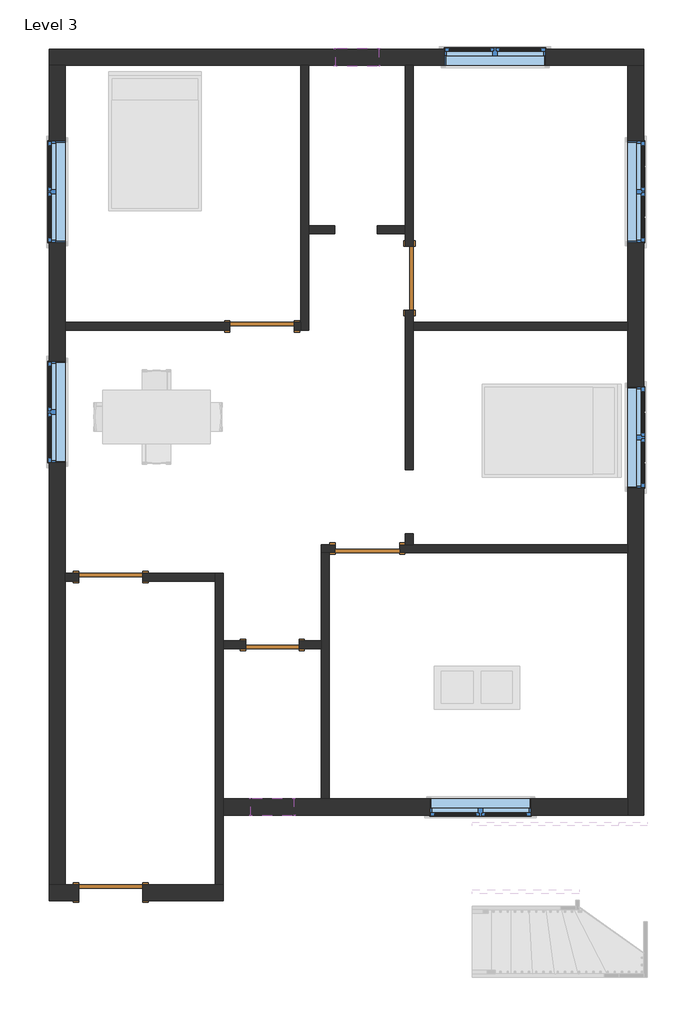
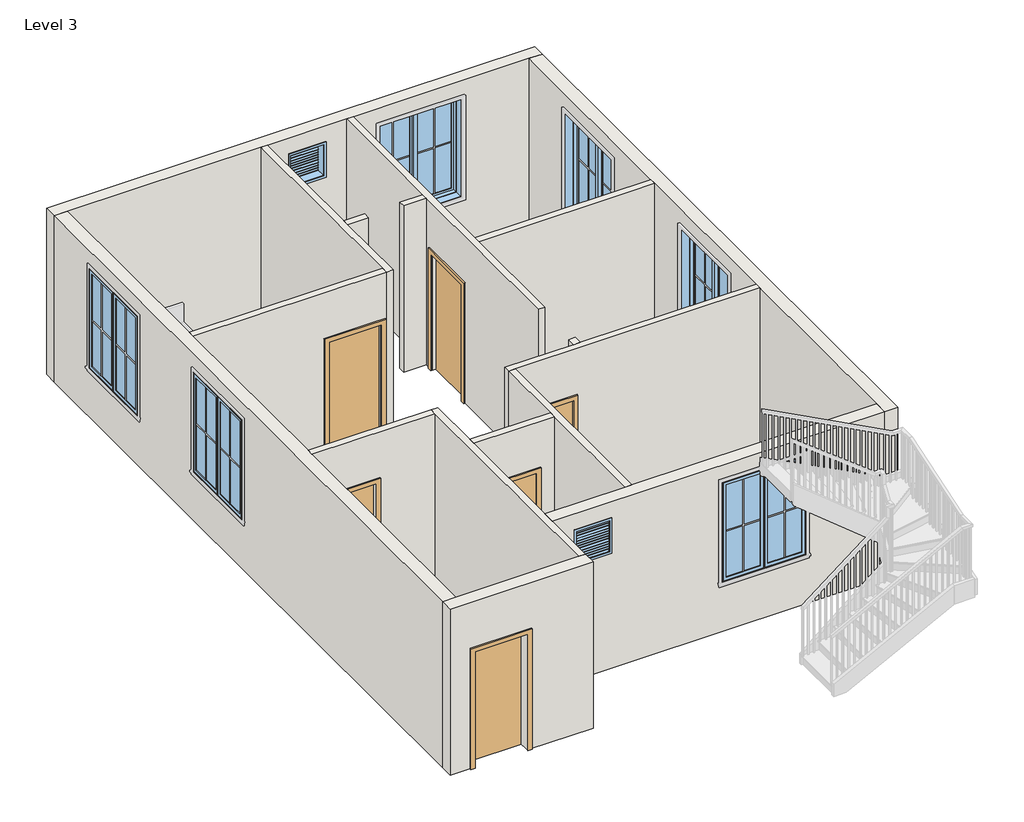
# One storey, part 1 of 3: 17 walls, 8 windows, 6 doors.
"""IFC4 building model written with IfcOpenShell, lengths in millimetres."""

from ifc_helpers import new_model, si_unit, frame, origin, place, context, project, spatial, polyline, outline, extrude, faceted_brep, transform, mapped, element, save
from components import door_214872d5, single_flush_door_3_e5f9f3c4, single_flush_door_3_305aa2a5, single_flush_door_3_a90ba1ad, window_9ac97e1a, window_f2d8fef0

model = new_model("IFC4")

# Units and contexts
model_context = context("Model", 3, world=origin())
ifc_project = project(units=[si_unit("LENGTHUNIT", "METRE", prefix="MILLI")], contexts=[model_context])

# Site, building, storey
site = spatial("IfcSite", under=ifc_project)
building = spatial("IfcBuilding", under=site)
storey = spatial("IfcBuildingStorey", under=building, Name="Level 3", Elevation=3200.4)

# Doors
placement = place(None, origin())
door_shape = door_214872d5(model_context)
element("IfcDoor", 1, ObjectType="Single-Flush : DOOR 2'6\"", at=placement, inside=storey, context=model_context, shape_type="MappedRepresentation", body=[
    mapped(door_shape, transform((-2309.3144966, -2885.2590409, 3200.4), x_axis=(-1.0, 0.0, 0.0), y_axis=(0.0, -1.0, 0.0), z_axis=(0.0, 0.0, 1.0))),
])
single_flush_door_3_shape = single_flush_door_3_e5f9f3c4(model_context)
element("IfcDoor", 2, ObjectType="Single-Flush : DOOR 3'", at=placement, inside=storey, context=model_context, shape_type="MappedRepresentation", body=[
    mapped(single_flush_door_3_shape, transform((-2455.3644966, 1648.6409591, 3200.4), x_axis=(1.0, 0.0, 0.0), y_axis=(0.0, 1.0, 0.0), z_axis=(0.0, 0.0, 1.0))),
])
element("IfcDoor", 3, ObjectType="Single-Flush : DOOR 3'", at=placement, inside=storey, context=model_context, shape_type="MappedRepresentation", body=[
    mapped(single_flush_door_3_shape, transform((-359.8644966, 2334.4409591, 3200.4), x_axis=(0.0, -1.0, 0.0), y_axis=(1.0, 0.0, 0.0), z_axis=(0.0, 0.0, 1.0))),
])
element("IfcDoor", 4, ObjectType="Single-Flush : DOOR 3'", at=placement, inside=storey, context=model_context, shape_type="MappedRepresentation", body=[
    mapped(single_flush_door_3_shape, transform((-956.7644966, -1513.6590409, 3200.4), x_axis=(-1.0, 0.0, 0.0), y_axis=(0.0, -1.0, 0.0), z_axis=(0.0, 0.0, 1.0))),
])
single_flush_door_3_2_shape = single_flush_door_3_305aa2a5(model_context)
element("IfcDoor", 5, ObjectType="Single-Flush : DOOR 3'", at=placement, inside=storey, context=model_context, shape_type="MappedRepresentation", body=[
    mapped(single_flush_door_3_2_shape, transform((-4608.0144966, -1920.0590409, 3200.4), x_axis=(-1.0, 0.0, 0.0), y_axis=(0.0, -1.0, 0.0), z_axis=(0.0, 0.0, 1.0))),
])
single_flush_door_3_3_shape = single_flush_door_3_a90ba1ad(model_context)
element("IfcDoor", 6, ObjectType="Single-Flush : DOOR 3'", at=placement, inside=storey, context=model_context, shape_type="MappedRepresentation", body=[
    mapped(single_flush_door_3_3_shape, transform((-4608.0144966, -6409.5090409, 3200.4), x_axis=(-1.0, 0.0, 0.0), y_axis=(0.0, -1.0, 0.0), z_axis=(0.0, 0.0, 1.0))),
])

# Walls
element("IfcWall", 7, ObjectType="WALL 4.5\"", at=placement, inside=storey, context=model_context, shape_type="Brep", body=[
    faceted_brep([(-1902.9144966, 5363.3909591, 3200.4), (-1902.9144966, 1705.7909591, 3200.4), (-1902.9144966, 1591.4909591, 3200.4), (-1902.9144966, 1591.4909591, 6248.4), (-1902.9144966, 1705.7909591, 6248.4), (-1902.9144966, 5363.3909591, 6248.4), (-1788.6144966, 5363.3909591, 3200.4), (-1788.6144966, 5363.3909591, 6248.4), (-1788.6144966, 3077.3909591, 6248.4), (-1788.6144966, 2963.0909591, 6248.4), (-1788.6144966, 1591.4909591, 6248.4), (-1788.6144966, 1591.4909591, 3200.4), (-1788.6144966, 2963.0909591, 3200.4), (-1788.6144966, 3077.3909591, 3200.4)], [[[0, 1, 2, 3, 4, 5]], [[6, 7, 8, 9, 10, 11, 12, 13]], [[2, 1, 0, 6, 13, 12, 11]], [[0, 5, 7, 6]], [[3, 2, 11, 10]], [[5, 4, 3, 10, 9, 8, 7]]]),
])
element("IfcWall", 8, ObjectType="WALL 4.5\"", at=placement, inside=storey, context=model_context, shape_type="SweptSolid", body=[
    extrude(outline(polyline([(5334.0, -1998.1644966), (3200.4, -1998.1644966), (3200.4, -1902.9144966), (6248.4, -1902.9144966), (6248.4, -5255.7144966), (3200.4, -5255.7144966), (3200.4, -2912.5644966), (5334.0, -2912.5644966), (5334.0, -1998.1644966)])), frame((0.0, 1591.4909591, 0.0), z_axis=(0.0, 1.0, 0.0), x_axis=(0.0, 0.0, 1.0)), (0.0, 0.0, 1.0), 114.3),
])
element("IfcWall", 9, ObjectType="WALL 4.5\"", at=placement, inside=storey, context=model_context, shape_type="Brep", body=[
    faceted_brep([(-417.0144966, 1877.2409591, 5334.0), (-417.0144966, 1877.2409591, 3200.4), (-417.0144966, -389.7090409, 3200.4), (-417.0144966, -389.7090409, 6248.4), (-417.0144966, 2963.0909591, 6248.4), (-417.0144966, 3077.3909591, 6248.4), (-417.0144966, 5363.3909591, 6248.4), (-417.0144966, 5363.3909591, 3200.4), (-417.0144966, 3077.3909591, 3200.4), (-417.0144966, 2963.0909591, 3200.4), (-417.0144966, 2791.6409591, 3200.4), (-417.0144966, 2791.6409591, 5334.0), (-302.7144966, -389.7090409, 3200.4), (-302.7144966, 1591.4909591, 3200.4), (-302.7144966, 1705.7909591, 3200.4), (-302.7144966, 1877.2409591, 3200.4), (-302.7144966, 1877.2409591, 5334.0), (-302.7144966, 2791.6409591, 5334.0), (-302.7144966, 2791.6409591, 3200.4), (-302.7144966, 5363.3909591, 3200.4), (-302.7144966, 5363.3909591, 6248.4), (-302.7144966, 1705.7909591, 6248.4), (-302.7144966, 1591.4909591, 6248.4), (-302.7144966, -389.7090409, 6248.4)], [[[0, 1, 2, 3, 4, 5, 6, 7, 8, 9, 10, 11]], [[12, 13, 14, 15, 16, 17, 18, 19, 20, 21, 22, 23]], [[2, 1, 15, 14, 13, 12]], [[10, 9, 8, 7, 19, 18]], [[3, 2, 12, 23]], [[7, 6, 20, 19]], [[16, 15, 1, 0]], [[17, 16, 0, 11]], [[18, 17, 11, 10]], [[6, 5, 4, 3, 23, 22, 21, 20]]]),
])
element("IfcWall", 10, ObjectType="WALL 4.5\"", at=placement, inside=storey, context=model_context, shape_type="SweptSolid", body=[
    extrude(outline(polyline([(-302.7144966, 1705.7909591), (2745.2855034, 1705.7909591), (2745.2855034, 1591.4909591), (-302.7144966, 1591.4909591), (-302.7144966, 1705.7909591)])), frame((0.0, 0.0, 3200.4), z_axis=(0.0, 0.0, 1.0), x_axis=(1.0, 0.0, 0.0)), (0.0, 0.0, 1.0), 3048.0),
])
element("IfcWall", 11, ObjectType="WALL 4.5\"", at=placement, inside=storey, context=model_context, shape_type="SweptSolid", body=[
    extrude(outline(polyline([(-1423.1234474, 2963.0909591), (-1788.6144966, 2963.0909591), (-1788.6144966, 3077.3909591), (-1423.1234474, 3077.3909591), (-1423.1234474, 2963.0909591)])), frame((0.0, 0.0, 3200.4), z_axis=(0.0, 0.0, 1.0), x_axis=(1.0, 0.0, 0.0)), (0.0, 0.0, 1.0), 3048.0),
])
element("IfcWall", 12, ObjectType="WALL 4.5\"", at=placement, inside=storey, context=model_context, shape_type="Brep", body=[
    faceted_brep([(-1413.9644966, -1456.5090409, 5334.0), (-1413.9644966, -1456.5090409, 3200.4), (-1610.8144966, -1456.5090409, 3200.4), (-1610.8144966, -1456.5090409, 6248.4), (-417.0144966, -1456.5090409, 6248.4), (-302.7144966, -1456.5090409, 6248.4), (2745.2855034, -1456.5090409, 6248.4), (2745.2855034, -1456.5090409, 3200.4), (-302.7144966, -1456.5090409, 3200.4), (-417.0144966, -1456.5090409, 3200.4), (-499.5644966, -1456.5090409, 3200.4), (-499.5644966, -1456.5090409, 5334.0), (-1610.8144966, -1570.8090409, 3200.4), (-1496.5144966, -1570.8090409, 3200.4), (-1413.9644966, -1570.8090409, 3200.4), (-1413.9644966, -1570.8090409, 5334.0), (-499.5644966, -1570.8090409, 5334.0), (-499.5644966, -1570.8090409, 3200.4), (2745.2855034, -1570.8090409, 3200.4), (2745.2855034, -1570.8090409, 6248.4), (-1496.5144966, -1570.8090409, 6248.4), (-1610.8144966, -1570.8090409, 6248.4)], [[[0, 1, 2, 3, 4, 5, 6, 7, 8, 9, 10, 11]], [[12, 13, 14, 15, 16, 17, 18, 19, 20, 21]], [[2, 1, 14, 13, 12]], [[10, 9, 8, 7, 18, 17]], [[7, 6, 19, 18]], [[3, 2, 12, 21]], [[15, 14, 1, 0]], [[16, 15, 0, 11]], [[17, 16, 11, 10]], [[6, 5, 4, 3, 21, 20, 19]]]),
])
element("IfcWall", 13, ObjectType="WALL 4.5\"", at=placement, inside=storey, context=model_context, shape_type="SweptSolid", body=[
    extrude(outline(polyline([(-302.7144966, -1304.1090409), (-302.7144966, -1456.5090409), (-417.0144966, -1456.5090409), (-417.0144966, -1304.1090409), (-302.7144966, -1304.1090409)])), frame((0.0, 0.0, 3200.4), z_axis=(0.0, 0.0, 1.0), x_axis=(1.0, 0.0, 0.0)), (0.0, 0.0, 1.0), 3048.0),
])
element("IfcWall", 14, ObjectType="WALL 4.5\"", at=placement, inside=storey, context=model_context, shape_type="Brep", body=[
    faceted_brep([(-1610.8144966, -1570.8090409, 3200.4), (-1610.8144966, -2828.1090409, 3200.4), (-1610.8144966, -2942.4090409, 3200.4), (-1610.8144966, -5076.0090409, 3200.4), (-1610.8144966, -5076.0090409, 6248.4), (-1610.8144966, -2942.4090409, 6248.4), (-1610.8144966, -2828.1090409, 6248.4), (-1610.8144966, -1570.8090409, 6248.4), (-1496.5144966, -1570.8090409, 3200.4), (-1496.5144966, -1570.8090409, 6248.4), (-1496.5144966, -5076.0090409, 6248.4), (-1496.5144966, -5076.0090409, 3200.4)], [[[0, 1, 2, 3, 4, 5, 6, 7]], [[8, 9, 10, 11]], [[3, 2, 1, 0, 8, 11]], [[0, 7, 9, 8]], [[4, 3, 11, 10]], [[7, 6, 5, 4, 10, 9]]]),
])
element("IfcWall", 15, ObjectType="WALL 4.5\"", at=placement, inside=storey, context=model_context, shape_type="SweptSolid", body=[
    extrude(outline(polyline([(3200.4, -3007.8144966), (3200.4, -2690.3144966), (5334.0, -2690.3144966), (5334.0, -1928.3144966), (3200.4, -1928.3144966), (3200.4, -1610.8144966), (6248.4, -1610.8144966), (6248.4, -3007.8144966), (3200.4, -3007.8144966)])), frame((0.0, -2942.4090409, 0.0), z_axis=(0.0, 1.0, 0.0), x_axis=(0.0, 0.0, 1.0)), (0.0, 0.0, 1.0), 114.3),
])
element("IfcWall", 16, ObjectType="WALL 4.5\"", at=placement, inside=storey, context=model_context, shape_type="Brep", body=[
    faceted_brep([(-3007.8144966, -6295.2090409, 3200.4), (-3007.8144966, -5304.6090409, 3200.4), (-3007.8144966, -5076.0090409, 3200.4), (-3007.8144966, -2942.4090409, 3200.4), (-3007.8144966, -2828.1090409, 3200.4), (-3007.8144966, -1862.9090409, 3200.4), (-3007.8144966, -1862.9090409, 6248.4), (-3007.8144966, -2828.1090409, 6248.4), (-3007.8144966, -2942.4090409, 6248.4), (-3007.8144966, -5076.0090409, 6248.4), (-3007.8144966, -5304.6090409, 6248.4), (-3007.8144966, -6295.2090409, 6248.4), (-3122.1144966, -6295.2090409, 3200.4), (-3122.1144966, -6295.2090409, 6248.4), (-3122.1144966, -1977.2090409, 6248.4), (-3122.1144966, -1862.9090409, 6248.4), (-3122.1144966, -1862.9090409, 3200.4), (-3122.1144966, -1977.2090409, 3200.4)], [[[0, 1, 2, 3, 4, 5, 6, 7, 8, 9, 10, 11]], [[12, 13, 14, 15, 16, 17]], [[5, 4, 3, 2, 1, 0, 12, 17, 16]], [[0, 11, 13, 12]], [[6, 5, 16, 15]], [[11, 10, 9, 8, 7, 6, 15, 14, 13]]]),
])
element("IfcWall", 17, ObjectType="WALL 4.5\"", at=placement, inside=storey, context=model_context, shape_type="SweptSolid", body=[
    extrude(outline(polyline([(3200.4, -5255.7144966), (3200.4, -5065.2144966), (5334.0, -5065.2144966), (5334.0, -4150.8144966), (3200.4, -4150.8144966), (3200.4, -3122.1144966), (6248.4, -3122.1144966), (6248.4, -5255.7144966), (3200.4, -5255.7144966)])), frame((0.0, -1977.2090409, 0.0), z_axis=(0.0, 1.0, 0.0), x_axis=(0.0, 0.0, 1.0)), (0.0, 0.0, 1.0), 114.3),
])
element("IfcWall", 18, ObjectType="WALL 4.5\"", at=placement, inside=storey, context=model_context, shape_type="SweptSolid", body=[
    extrude(outline(polyline([(-417.0144966, 2963.0909591), (-814.3659123, 2963.0909591), (-814.3659123, 3077.3909591), (-417.0144966, 3077.3909591), (-417.0144966, 2963.0909591)])), frame((0.0, 0.0, 3200.4), z_axis=(0.0, 0.0, 1.0), x_axis=(1.0, 0.0, 0.0)), (0.0, 0.0, 1.0), 3048.0),
])
element("IfcWall", 19, ObjectType="WALL 9\"", at=placement, inside=storey, context=model_context, shape_type="Brep", body=[
    faceted_brep([(-5484.3144966, 5363.3909591, 3200.4), (-5255.7144966, 5363.3909591, 3200.4), (-1902.9144966, 5363.3909591, 3200.4), (-1788.6144966, 5363.3909591, 3200.4), (-417.0144966, 5363.3909591, 3200.4), (-302.7144966, 5363.3909591, 3200.4), (2745.2855034, 5363.3909591, 3200.4), (2973.8855034, 5363.3909591, 3200.4), (2973.8855034, 5363.3909591, 6248.4), (2745.2855034, 5363.3909591, 6248.4), (-302.7144966, 5363.3909591, 6248.4), (-417.0144966, 5363.3909591, 6248.4), (-1788.6144966, 5363.3909591, 6248.4), (-1902.9144966, 5363.3909591, 6248.4), (-5255.7144966, 5363.3909591, 6248.4), (-5484.3144966, 5363.3909591, 6248.4), (1583.2355034, 5363.3909591, 5943.6), (1583.2355034, 5363.3909591, 4114.8), (135.4355034, 5363.3909591, 4114.8), (135.4355034, 5363.3909591, 5943.6), (-1407.6144966, 5363.3909591, 5943.6), (-798.0144966, 5363.3909591, 5943.6), (-798.0144966, 5363.3909591, 5334.0), (-1407.6144966, 5363.3909591, 5334.0), (-5484.3144966, 5591.9909591, 3200.4), (-5484.3144966, 5591.9909591, 6248.4), (2973.8855034, 5591.9909591, 6248.4), (2973.8855034, 5591.9909591, 3200.4), (1583.2355034, 5591.9909591, 5943.6), (135.4355034, 5591.9909591, 5943.6), (135.4355034, 5591.9909591, 4114.8), (1583.2355034, 5591.9909591, 4114.8), (-1407.6144966, 5591.9909591, 5943.6), (-1407.6144966, 5591.9909591, 5334.0), (-798.0144966, 5591.9909591, 5334.0), (-798.0144966, 5591.9909591, 5943.6)], [[[0, 1, 2, 3, 4, 5, 6, 7, 8, 9, 10, 11, 12, 13, 14, 15], [16, 17, 18, 19], [20, 21, 22, 23]], [[24, 25, 26, 27], [28, 29, 30, 31], [32, 33, 34, 35]], [[7, 6, 5, 4, 3, 2, 1, 0, 24, 27]], [[8, 7, 27, 26]], [[0, 15, 25, 24]], [[17, 16, 28, 31]], [[18, 17, 31, 30]], [[19, 18, 30, 29]], [[16, 19, 29, 28]], [[33, 32, 20, 23]], [[34, 33, 23, 22]], [[35, 34, 22, 21]], [[32, 35, 21, 20]], [[15, 14, 13, 12, 11, 10, 9, 8, 26, 25]]]),
])
element("IfcWall", 20, ObjectType="WALL 9\"", at=placement, inside=storey, context=model_context, shape_type="Brep", body=[
    faceted_brep([(2745.2855034, 5363.3909591, 3200.4), (2745.2855034, 1705.7909591, 3200.4), (2745.2855034, 1591.4909591, 3200.4), (2745.2855034, -1456.5090409, 3200.4), (2745.2855034, -1570.8090409, 3200.4), (2745.2855034, -5076.0090409, 3200.4), (2745.2855034, -5304.6090409, 3200.4), (2745.2855034, -5304.6090409, 6248.4), (2745.2855034, -5076.0090409, 6248.4), (2745.2855034, -1570.8090409, 6248.4), (2745.2855034, -1456.5090409, 6248.4), (2745.2855034, 1591.4909591, 6248.4), (2745.2855034, 1705.7909591, 6248.4), (2745.2855034, 5363.3909591, 6248.4), (2745.2855034, -656.4090409, 5943.6), (2745.2855034, -656.4090409, 4114.8), (2745.2855034, 791.3909591, 4114.8), (2745.2855034, 791.3909591, 5943.6), (2745.2855034, 2839.2659591, 5943.6), (2745.2855034, 2839.2659591, 4114.8), (2745.2855034, 4287.0659591, 4114.8), (2745.2855034, 4287.0659591, 5943.6), (2973.8855034, 5363.3909591, 3200.4), (2973.8855034, 5363.3909591, 6248.4), (2973.8855034, -5304.6090409, 6248.4), (2973.8855034, -5304.6090409, 3200.4), (2973.8855034, -656.4090409, 5943.6), (2973.8855034, 791.3909591, 5943.6), (2973.8855034, 791.3909591, 4114.8), (2973.8855034, -656.4090409, 4114.8), (2973.8855034, 2839.2659591, 5943.6), (2973.8855034, 4287.0659591, 5943.6), (2973.8855034, 4287.0659591, 4114.8), (2973.8855034, 2839.2659591, 4114.8)], [[[0, 1, 2, 3, 4, 5, 6, 7, 8, 9, 10, 11, 12, 13], [14, 15, 16, 17], [18, 19, 20, 21]], [[22, 23, 24, 25], [26, 27, 28, 29], [30, 31, 32, 33]], [[6, 5, 4, 3, 2, 1, 0, 22, 25]], [[0, 13, 23, 22]], [[7, 6, 25, 24]], [[15, 14, 26, 29]], [[16, 15, 29, 28]], [[17, 16, 28, 27]], [[14, 17, 27, 26]], [[19, 18, 30, 33]], [[20, 19, 33, 32]], [[21, 20, 32, 31]], [[18, 21, 31, 30]], [[13, 12, 11, 10, 9, 8, 7, 24, 23]]]),
])
element("IfcWall", 21, ObjectType="WALL 9\"", at=placement, inside=storey, context=model_context, shape_type="Brep", body=[
    faceted_brep([(2745.2855034, -5076.0090409, 3200.4), (-1496.5144966, -5076.0090409, 3200.4), (-1610.8144966, -5076.0090409, 3200.4), (-3007.8144966, -5076.0090409, 3200.4), (-3007.8144966, -5076.0090409, 6248.4), (-1610.8144966, -5076.0090409, 6248.4), (-1496.5144966, -5076.0090409, 6248.4), (2745.2855034, -5076.0090409, 6248.4), (-70.9394966, -5076.0090409, 5943.6), (-70.9394966, -5076.0090409, 4114.8), (1376.8605034, -5076.0090409, 4114.8), (1376.8605034, -5076.0090409, 5943.6), (-2004.5144966, -5076.0090409, 5943.6), (-2614.1144966, -5076.0090409, 5943.6), (-2614.1144966, -5076.0090409, 5334.0), (-2004.5144966, -5076.0090409, 5334.0), (2745.2855034, -5304.6090409, 3200.4), (2745.2855034, -5304.6090409, 6248.4), (-3007.8144966, -5304.6090409, 6248.4), (-3007.8144966, -5304.6090409, 3200.4), (-70.9394966, -5304.6090409, 5943.6), (1376.8605034, -5304.6090409, 5943.6), (1376.8605034, -5304.6090409, 4114.8), (-70.9394966, -5304.6090409, 4114.8), (-2004.5144966, -5304.6090409, 5943.6), (-2004.5144966, -5304.6090409, 5334.0), (-2614.1144966, -5304.6090409, 5334.0), (-2614.1144966, -5304.6090409, 5943.6)], [[[0, 1, 2, 3, 4, 5, 6, 7], [8, 9, 10, 11], [12, 13, 14, 15]], [[16, 17, 18, 19], [20, 21, 22, 23], [24, 25, 26, 27]], [[3, 2, 1, 0, 16, 19]], [[0, 7, 17, 16]], [[4, 3, 19, 18]], [[9, 8, 20, 23]], [[10, 9, 23, 22]], [[11, 10, 22, 21]], [[8, 11, 21, 20]], [[25, 24, 12, 15]], [[26, 25, 15, 14]], [[27, 26, 14, 13]], [[24, 27, 13, 12]], [[7, 6, 5, 4, 18, 17]]]),
])
element("IfcWall", 22, ObjectType="WALL 9\"", at=placement, inside=storey, context=model_context, shape_type="Brep", body=[
    faceted_brep([(-5065.2144966, -6295.2090409, 5334.0), (-5065.2144966, -6295.2090409, 3200.4), (-5255.7144966, -6295.2090409, 3200.4), (-5484.3144966, -6295.2090409, 3200.4), (-5484.3144966, -6295.2090409, 6248.4), (-5255.7144966, -6295.2090409, 6248.4), (-3122.1144966, -6295.2090409, 6248.4), (-3007.8144966, -6295.2090409, 6248.4), (-3007.8144966, -6295.2090409, 3200.4), (-3122.1144966, -6295.2090409, 3200.4), (-4150.8144966, -6295.2090409, 3200.4), (-4150.8144966, -6295.2090409, 5334.0), (-5484.3144966, -6523.8090409, 3200.4), (-5065.2144966, -6523.8090409, 3200.4), (-5065.2144966, -6523.8090409, 5334.0), (-4150.8144966, -6523.8090409, 5334.0), (-4150.8144966, -6523.8090409, 3200.4), (-3007.8144966, -6523.8090409, 3200.4), (-3007.8144966, -6523.8090409, 6248.4), (-5484.3144966, -6523.8090409, 6248.4)], [[[0, 1, 2, 3, 4, 5, 6, 7, 8, 9, 10, 11]], [[12, 13, 14, 15, 16, 17, 18, 19]], [[10, 9, 8, 17, 16]], [[3, 2, 1, 13, 12]], [[4, 3, 12, 19]], [[8, 7, 18, 17]], [[7, 6, 5, 4, 19, 18]], [[14, 13, 1, 0]], [[15, 14, 0, 11]], [[16, 15, 11, 10]]]),
])
element("IfcWall", 23, ObjectType="WALL 9\"", at=placement, inside=storey, context=model_context, shape_type="Brep", body=[
    faceted_brep([(-5255.7144966, -6295.2090409, 3200.4), (-5255.7144966, -1977.2090409, 3200.4), (-5255.7144966, -1862.9090409, 3200.4), (-5255.7144966, 1591.4909591, 3200.4), (-5255.7144966, 1705.7909591, 3200.4), (-5255.7144966, 5363.3909591, 3200.4), (-5255.7144966, 5363.3909591, 6248.4), (-5255.7144966, 1705.7909591, 6248.4), (-5255.7144966, 1591.4909591, 6248.4), (-5255.7144966, -1862.9090409, 6248.4), (-5255.7144966, -1977.2090409, 6248.4), (-5255.7144966, -6295.2090409, 6248.4), (-5255.7144966, 4287.0659591, 5943.6), (-5255.7144966, 4287.0659591, 4114.8), (-5255.7144966, 2839.2659591, 4114.8), (-5255.7144966, 2839.2659591, 5943.6), (-5255.7144966, 1153.3409591, 5943.6), (-5255.7144966, 1153.3409591, 4114.8), (-5255.7144966, -294.4590409, 4114.8), (-5255.7144966, -294.4590409, 5943.6), (-5484.3144966, -6295.2090409, 3200.4), (-5484.3144966, -6295.2090409, 6248.4), (-5484.3144966, 5363.3909591, 6248.4), (-5484.3144966, 5363.3909591, 3200.4), (-5484.3144966, 4287.0659591, 5943.6), (-5484.3144966, 2839.2659591, 5943.6), (-5484.3144966, 2839.2659591, 4114.8), (-5484.3144966, 4287.0659591, 4114.8), (-5484.3144966, 1153.3409591, 5943.6), (-5484.3144966, -294.4590409, 5943.6), (-5484.3144966, -294.4590409, 4114.8), (-5484.3144966, 1153.3409591, 4114.8)], [[[0, 1, 2, 3, 4, 5, 6, 7, 8, 9, 10, 11], [12, 13, 14, 15], [16, 17, 18, 19]], [[20, 21, 22, 23], [24, 25, 26, 27], [28, 29, 30, 31]], [[5, 4, 3, 2, 1, 0, 20, 23]], [[0, 11, 21, 20]], [[6, 5, 23, 22]], [[13, 12, 24, 27]], [[14, 13, 27, 26]], [[15, 14, 26, 25]], [[12, 15, 25, 24]], [[17, 16, 28, 31]], [[18, 17, 31, 30]], [[19, 18, 30, 29]], [[16, 19, 29, 28]], [[11, 10, 9, 8, 7, 6, 22, 21]]]),
])

# Windows
window_shape = window_9ac97e1a(model_context)
element("IfcWindow", 24, ObjectType="Window-Casement-Double : 57\" x 72\"", at=placement, inside=storey, context=model_context, shape_type="MappedRepresentation", body=[
    mapped(window_shape, transform((2859.5855034, 67.4909591, 3200.4), x_axis=(0.0, -1.0, 0.0), y_axis=(1.0, 0.0, 0.0), z_axis=(0.0, 0.0, 1.0))),
])
element("IfcWindow", 25, ObjectType="Window-Casement-Double : 57\" x 72\"", at=placement, inside=storey, context=model_context, shape_type="MappedRepresentation", body=[
    mapped(window_shape, transform((2859.5855034, 3563.1659591, 3200.4), x_axis=(0.0, -1.0, 0.0), y_axis=(1.0, 0.0, 0.0), z_axis=(0.0, 0.0, 1.0))),
])
element("IfcWindow", 26, ObjectType="Window-Casement-Double : 57\" x 72\"", at=placement, inside=storey, context=model_context, shape_type="MappedRepresentation", body=[
    mapped(window_shape, transform((859.3355034, 5477.6909591, 3200.4), x_axis=(1.0, 0.0, 0.0), y_axis=(0.0, 1.0, 0.0), z_axis=(0.0, 0.0, 1.0))),
])
element("IfcWindow", 27, ObjectType="Window-Casement-Double : 57\" x 72\"", at=placement, inside=storey, context=model_context, shape_type="MappedRepresentation", body=[
    mapped(window_shape, transform((-5370.0144966, 3563.1659591, 3200.4), x_axis=(0.0, 1.0, 0.0), y_axis=(-1.0, 0.0, 0.0), z_axis=(0.0, 0.0, 1.0))),
])
element("IfcWindow", 28, ObjectType="Window-Casement-Double : 57\" x 72\"", at=placement, inside=storey, context=model_context, shape_type="MappedRepresentation", body=[
    mapped(window_shape, transform((-5370.0144966, 429.4409591, 3200.4), x_axis=(0.0, 1.0, 0.0), y_axis=(-1.0, 0.0, 0.0), z_axis=(0.0, 0.0, 1.0))),
])
element("IfcWindow", 29, ObjectType="Window-Casement-Double : 57\" x 72\"", at=placement, inside=storey, context=model_context, shape_type="MappedRepresentation", body=[
    mapped(window_shape, transform((652.9605034, -5190.3090409, 3200.4), x_axis=(-1.0, 0.0, 0.0), y_axis=(0.0, -1.0, 0.0), z_axis=(0.0, 0.0, 1.0))),
])
window_2_shape = window_f2d8fef0(model_context)
element("IfcWindow", 30, ObjectType="Window-Louvers : 24\" x 24\"", at=placement, inside=storey, context=model_context, shape_type="MappedRepresentation", body=[
    mapped(window_2_shape, transform((-1102.8144966, 5484.0409591, 4419.6), x_axis=(1.0, 0.0, 0.0), y_axis=(0.0, 1.0, 0.0), z_axis=(0.0, 0.0, 1.0))),
])
element("IfcWindow", 31, ObjectType="Window-Louvers : 24\" x 24\"", at=placement, inside=storey, context=model_context, shape_type="MappedRepresentation", body=[
    mapped(window_2_shape, transform((-2309.3144966, -5196.6590409, 4419.6), x_axis=(-1.0, 0.0, 0.0), y_axis=(0.0, -1.0, 0.0), z_axis=(0.0, 0.0, 1.0))),
])

save(model, "model.ifc")

# Revit data of these elements
# Type "Single-Flush : DOOR 2'6\""
#   Type Mark = "10"
#   Construction Type Id = "MDOOR"
#   Assembly Code = "C1020"
#   Analytic Construction = "Metal"
#   Thickness = 0' - 2"
#   Heat Transfer Coefficient (U) = 0.651978 BTU/(h·ft²·°F)
#   Height = 7' - 0"
#   Trim Projection Ext = 0' - 1"
#   Trim Projection Int = 0' - 1"
#   Trim Width = 0' - 3"
#   Width = 2' - 6"
#   Define Thermal Properties by = 1
#   Door Material = Door - Panel
#   Frame Material = Door - Frame
#   Visual Light Transmittance = 0
#   Solar Heat Gain Coefficient = 0
#   Function = (empty or 0)
#   Wall Closure = (empty or 0)
# Type "Single-Flush : DOOR 3'"
#   Type Mark = "9"
#   Construction Type Id = "MDOOR"
#   Assembly Code = "C1020"
#   Analytic Construction = "Metal"
#   Thickness = 0' - 2"
#   Heat Transfer Coefficient (U) = 0.651978 BTU/(h·ft²·°F)
#   Height = 7' - 0"
#   Trim Projection Ext = 0' - 1"
#   Trim Projection Int = 0' - 1"
#   Trim Width = 0' - 3"
#   Width = 3' - 0"
#   Define Thermal Properties by = 1
#   Door Material = Door - Panel
#   Frame Material = Door - Frame
#   Visual Light Transmittance = 0
#   Solar Heat Gain Coefficient = 0
#   Function = (empty or 0)
#   Wall Closure = (empty or 0)
# Type "WALL 4.5\""
#   Assembly Code = "B2010"
#   Layers, outside or top first: 0' - 4 1/2" no material (function 1)
# Type "WALL 9\""
#   Assembly Code = "B2010"
#   Layers, outside or top first: 0' - 9" no material (function 1)
# Type "Window-Casement-Double : 57\" x 72\""
#   Type Mark = "17"
#   Fire Rating = "0.5h"
#   Assembly Code = "B2020100"
#   Analytic Construction = "Double glazing - domestic"
#   Frame Extension [instance default] = 0' - 0 1/4"
#   Window Inset [instance default] = 0' - 0"
#   Wall Thickness [instance default] = 0' - 6"
#   Interior Wall Closure [instance default] = 0' - 2 1/4"
#   Half Width = 2' - 4 1/2"
#   Visual Light Transmittance = 0.81
#   Thermal Resistance (R) = 1.8146 (h·ft²·°F)/BTU
#   Solar Heat Gain Coefficient = 0.76
#   Rough Width = 4' - 9 1/2"
#   Rough Height = 6' - 0 1/2"
#   Height = 6' - 0"
#   Heat Transfer Coefficient (U) = 0.5511 BTU/(h·ft²·°F)
#   Exterior Wall Closure [instance default] = 0' - 1 1/4"
#   Extension Jamb [instance default] = 0' - 2 1/4"
#   Default Sill Height = 3' - 0"
#   Width = 4' - 9"
#   Define Thermal Properties by = 0
#   Muntin Visibility = yes
#   Interior Trim Visibility [instance default] = yes
#   Exterior Trim Visibility [instance default] = yes
#   Extension Jamb Visibility [instance default] = yes
#   Interior Trim Material = Wood - Stained
#   Muntin Pattern = Muntin Pattern_2x2 : Muntin Pattern_2x2
#   Interior Trim = Trim-Window-Interior-Flat : Picture Frame
#   Interior Frame Material = Wood - Stained
#   Glass Panel Material = Glass
#   Exterior Trim Material = Clad - White
#   Exterior Trim = Trim-Window-Exterior-Flat : with Sill
#   Exterior Frame Material = Clad - White
#   Wall Closure = (empty or 0)
# Type "Window-Louvers : 24\" x 24\""
#   Type Mark = "18"
#   Construction Type Id = "GSP4R"
#   Assembly Code = "B20"
#   Analytic Construction = "1/8 in Pilkington single glazing"
#   Visual Light Transmittance = 0.9
#   Thermal Resistance (R) = 1.53941 (h·ft²·°F)/BTU
#   Solar Heat Gain Coefficient = 0.78
#   Max Height = 1' - 11.74264"
#   Height = 2' - 0"
#   Heat Transfer Coefficient (U) = 0.6496 BTU/(h·ft²·°F)
#   Blade Width [instance default] = 1' - 10 1/2"
#   Blade Vertical Thickness = 0' - 0.35355"
#   Blade Thickness = 0' - 0 1/4"
#   Blade Spacing = 0' - 1 1/2"
#   Blade Height = 0' - 1.85355"
#   Blade Depth = 0' - 3"
#   Blade Angle = 45.00°
#   Default Sill Height = 3' - 0"
#   Trim Projection_Exterior = 0' - 0 1/2"
#   Trim Projection_Interior = 0' - 0 1/2"
#   Trim Width_Exterior = 0' - 1 1/2"
#   Trim Width_Interior = 0' - 1 1/2"
#   Width = 2' - 0"
#   Max Blade Count = 12
#   Define Thermal Properties by = 1
#   Blade Count = 12
#   Frame Material = Birch
#   Louver Material = Birch
#   Trim Exterior Material = Birch
#   Trim Interior Material = Birch
#   Wall Closure = (empty or 0)
# Element 1 (IfcDoor, "Single-Flush : DOOR 2'6\"")
#   Phase Created = New Construction
#   Materials on its faces: "Door - Frame", "Door - Panel"
# Elements 2, 3, 4, 5, 6 (IfcDoor, "Single-Flush : DOOR 3'")
#   Phase Created = New Construction
#   Materials on its faces: "Door - Frame", "Door - Panel"
# Elements 7, 8, 9, 10, 11, 12, 13, 14, 15, 16, 17, 18 (IfcWall, "WALL 4.5\"")
#   Top Offset = 0' - 0"
#   Base Offset = 0' - 0"
#   Unconnected Height = 10' - 0"
#   wall height = 10' - 0"
#   Phase Created = New Construction
#   Base Constraint = Level 3
#   Materials on its faces: "Default Wall"
# Elements 19, 20, 21, 22, 23 (IfcWall, "WALL 9\"")
#   Top Offset = 0' - 0"
#   Base Offset = 0' - 0"
#   Unconnected Height = 10' - 0"
#   wall height = 10' - 0"
#   Phase Created = New Construction
#   Base Constraint = Level 3
#   Materials on its faces: "Default Wall"
# Element 24 (IfcWindow, "Window-Casement-Double : 57\" x 72\"")
#   Mark = "9"
#   Window Inset = 0' - 0"
#   Interior Wall Closure = 0' - 2 1/4"
#   Frame Extension = 0' - 0 1/4"
#   Exterior Wall Closure = 0' - 1 1/4"
#   Interior Trim Visibility = yes
#   Exterior Trim Visibility = yes
#   Phase Created = New Construction
#   Materials on its faces: "Wood - Stained", "Glass", "Clad - White"
# Element 25 (IfcWindow, "Window-Casement-Double : 57\" x 72\"")
#   Mark = "10"
#   Window Inset = 0' - 0"
#   Interior Wall Closure = 0' - 2 1/4"
#   Frame Extension = 0' - 0 1/4"
#   Exterior Wall Closure = 0' - 1 1/4"
#   Interior Trim Visibility = yes
#   Exterior Trim Visibility = yes
#   Phase Created = New Construction
#   Materials on its faces: "Wood - Stained", "Glass", "Clad - White"
# Element 26 (IfcWindow, "Window-Casement-Double : 57\" x 72\"")
#   Mark = "11"
#   Window Inset = 0' - 0"
#   Interior Wall Closure = 0' - 2 1/4"
#   Frame Extension = 0' - 0 1/4"
#   Exterior Wall Closure = 0' - 1 1/4"
#   Interior Trim Visibility = yes
#   Exterior Trim Visibility = yes
#   Phase Created = New Construction
#   Materials on its faces: "Wood - Stained", "Glass", "Clad - White"
# Element 27 (IfcWindow, "Window-Casement-Double : 57\" x 72\"")
#   Mark = "12"
#   Window Inset = 0' - 0"
#   Interior Wall Closure = 0' - 2 1/4"
#   Frame Extension = 0' - 0 1/4"
#   Exterior Wall Closure = 0' - 1 1/4"
#   Interior Trim Visibility = yes
#   Exterior Trim Visibility = yes
#   Phase Created = New Construction
#   Materials on its faces: "Wood - Stained", "Glass", "Clad - White"
# Element 28 (IfcWindow, "Window-Casement-Double : 57\" x 72\"")
#   Mark = "13"
#   Window Inset = 0' - 0"
#   Interior Wall Closure = 0' - 2 1/4"
#   Frame Extension = 0' - 0 1/4"
#   Exterior Wall Closure = 0' - 1 1/4"
#   Interior Trim Visibility = yes
#   Exterior Trim Visibility = yes
#   Phase Created = New Construction
#   Materials on its faces: "Wood - Stained", "Glass", "Clad - White"
# Element 29 (IfcWindow, "Window-Casement-Double : 57\" x 72\"")
#   Mark = "14"
#   Window Inset = 0' - 0"
#   Interior Wall Closure = 0' - 2 1/4"
#   Frame Extension = 0' - 0 1/4"
#   Exterior Wall Closure = 0' - 1 1/4"
#   Interior Trim Visibility = yes
#   Exterior Trim Visibility = yes
#   Phase Created = New Construction
#   Materials on its faces: "Wood - Stained", "Glass", "Clad - White"
# Element 30 (IfcWindow, "Window-Louvers : 24\" x 24\"")
#   Mark = "15"
#   Blade Width = 1' - 10 1/2"
#   Phase Created = New Construction
#   Materials on its faces: "Birch"
# Element 31 (IfcWindow, "Window-Louvers : 24\" x 24\"")
#   Mark = "16"
#   Blade Width = 1' - 10 1/2"
#   Phase Created = New Construction
#   Materials on its faces: "Birch"
# Materials
#   "Door - Panel": class "Wood", colour RGB 210 159 95, transparency 0, Cost = 0
#   "Door - Frame": colour RGB 118 70 51, transparency 0, Cost = 0
#   "Wood - Stained": class "Wood", colour RGB 224 178 126, transparency 0, Cost = 0
#   "Glass": class "Glass", colour RGB 0 128 192, transparency 0.75, Description = "Soda Lime Glass", Cost = 0
#   "Clad - White": class "Wood", colour RGB 242 242 238, transparency 0, Cost = 0
#   "Birch": class "Wood", colour RGB 224 178 126, transparency 0, Description = "Betula Alleghaniensis", Cost = 0
#   "Default Wall": colour RGB 128 128 128, transparency 0, Cost = 0
